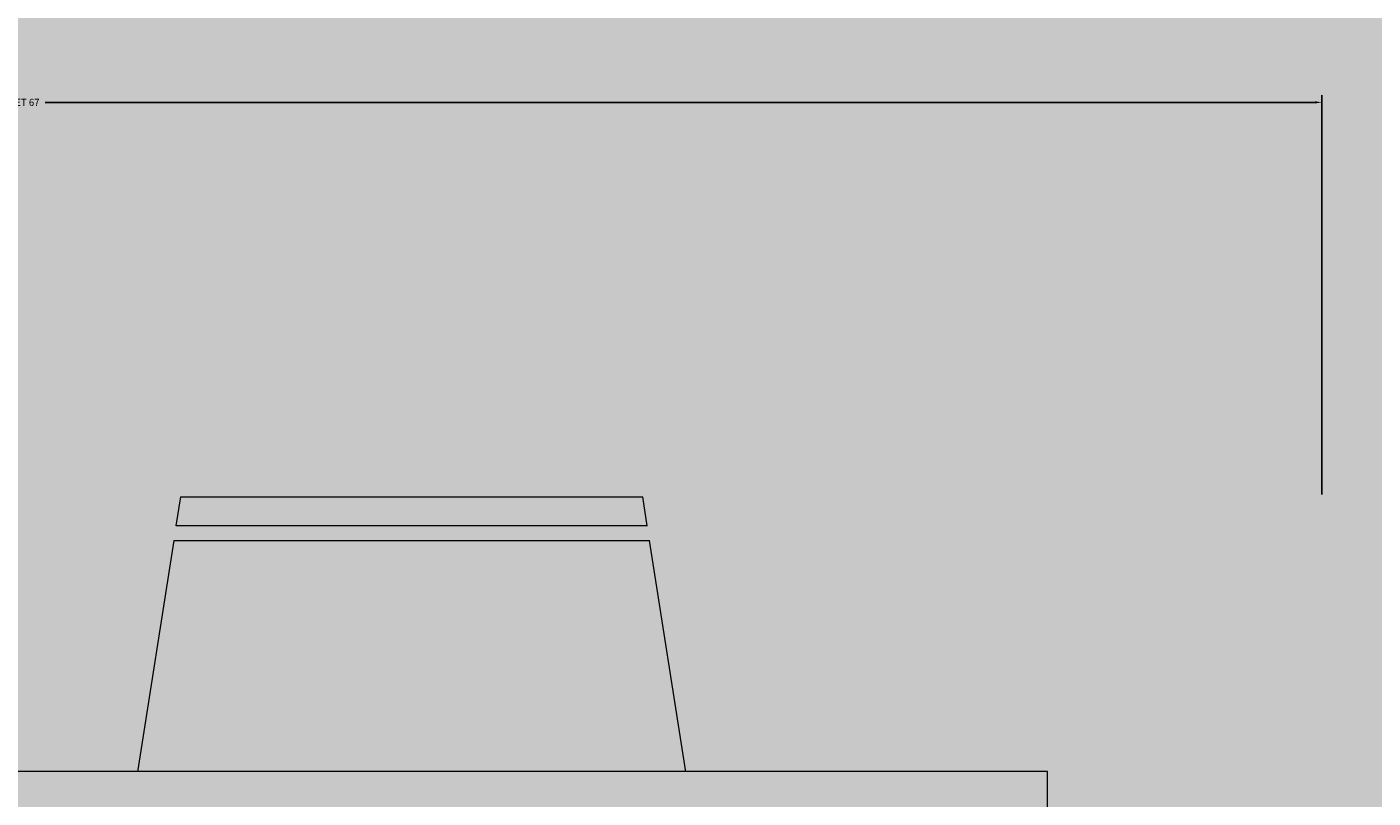
# Model space of a CAD drawing. Units: inches. Extents: x 3024 to 3952, y 1308 to 1863.
# Tile 12 of 29: x 3357 to 3392, y 1613 to 1633. Entities that reach past the tile are written whole.
import ezdxf

# ---------------------------------------------------------------- set-up
doc = ezdxf.new("R2010")
doc.units = ezdxf.units.IN
for name, color, linetype, lineweight in [('A-ANNO-DIMS', 2, 'Continuous', 18), ('A-FLOR-TILE-PATT', 7, 'Continuous', 13), ('A-FURN', 8, 'Continuous', 18), ('A-FURN-PATT', 9, 'Continuous', 13)]:
    doc.layers.add(name, color=color, linetype=linetype, lineweight=lineweight)
doc.layers.add('A-FLOR-PATT', color=254, linetype='Continuous', lineweight=13, true_color=0xfeeab9)
doc.styles.get("Standard").update_dxf_attribs({"font": 'arial.ttf'})
doc.dimstyles.get("Standard").update_dxf_attribs({"dimtxt": 0.18, "dimasz": 0.18, "dimexe": 0.18, "dimexo": 0.0625, "dimgap": 0.09, "dimtad": 0, "dimtih": 1, "dimtoh": 1, "dimdec": 4, "dimzin": 0, "dimdsep": 46, "dimtxsty": 'Standard', "dimcen": 0.09, "dimadec": 0, "dimazin": 0, "dimtfac": 1, "dimtdec": 4, "dimtofl": 0, "dimtmove": 0, "dimatfit": 3, "dimfxl": 1, "dimtolj": 1, "dimtzin": 0, "dimarcsym": 0})

# ---------------------------------------------------------------- blocks, each defined once
blk = doc.blocks.new('Dining Set - 36 x 72 in.')
for p, q in [((6, 27.5), (5.8438, 26.50042)), ((6, 27.5), (22, 27.5)), ((22.1563, 26.49966), (22, 27.5)), ((22.1584, 26.5), (5.8466, 26.5)), ((5.7657, 26.00059), (4.5153, 17.99762)), ((5.7696, 26), (22.2392, 26)), ((23.4848, 17.99762), (22.2345, 25.99926)), ((36, 18), (-36, 18)), ((36, -18), (36, 18))]:
    blk.add_line(p, q)
blk = doc.blocks.new('*D20')
at = {"layer": 'A-ANNO-DIMS', "color": 0, "lineweight": -2, "transparency": 16777216}
for p, q in [((3323.117, 1621.176), (3323.117, 1631.358)), ((3323.297, 1631.178), (3355.696, 1631.178)), ((3390.032, 1631.178), (3357.634, 1631.178)), ((3390.212, 1621.176), (3390.212, 1631.358))]:
    blk.add_line(p, q, dxfattribs=at)
at = {"layer": 'A-ANNO-DIMS', "color": 0, "transparency": 16777216}
for points in [[(3323.297, 1631.208), (3323.297, 1631.148), (3323.117, 1631.178)], [(3390.032, 1631.208), (3390.032, 1631.148), (3390.212, 1631.178)]]:
    blk.add_solid(points, dxfattribs=at)
at = {"layer": 'Defpoints', "color": 0, "transparency": 16777216}
for p in [(3390.212, 1631.178), (3323.117, 1621.114), (3390.212, 1621.114)]:
    blk.add_point(p, dxfattribs=at)
at = {"layer": 'A-ANNO-DIMS', "color": 0, "transparency": 16777216, "insert": (3356.665, 1631.178), "char_height": 0.18, "attachment_point": 5}
blk.add_mtext('\\A1;DINING SET 67', dxfattribs=at)

msp = doc.modelspace()

# ---------------------------------------------------------------- hatches: boundary and pattern name
at = {"layer": 'A-FLOR-PATT', "transparency": 33554528}
h = msp.add_hatch(color=256, dxfattribs=at)
h.dxf.hatch_style = 1
h.paths.add_polyline_path([(3460.764, 1688.6064), (3412.764, 1688.6064), (3412.764, 1694.6064), (3460.764, 1694.6064), (3460.764, 1778.6064), (3406.764, 1778.6064), (3406.764, 1759.9514), (3318.2981, 1759.9514), (3318.2981, 1658.6064), (3322.5356, 1658.6064), (3322.5356, 1652.6064), (3292.764, 1652.6064), (3292.764, 1778.6064), (3106.764, 1778.6064), (3106.764, 1628.6064), (3172.764, 1628.6064), (3172.764, 1532.6064), (3166.764, 1532.6064), (3166.764, 1628.6064), (3106.764, 1628.6064), (3106.764, 1356.8452), (3202.812, 1356.8452), (3202.812, 1354.2534), (3202.812, 1353.8388), (3202.812, 1351.1212), (3202.812, 1347.8452), (3277.764, 1347.8452), (3277.764, 1353.8452), (3277.764, 1356.8452), (3277.764, 1442.6064), (3460.764, 1442.6064)])
h.paths.add_polyline_path([(3216.238, 1527.2064), (3216.238, 1491.2064), (3214.663, 1491.2064), (3214.663, 1491.2409, -0.3966224), (3180.243, 1526.6064), (3163.0285, 1526.6064), (3163.0285, 1531.1064), (3161.716, 1531.1064), (3161.716, 1561.1064), (3163.0285, 1561.1064), (3163.0285, 1531.1064), (3163.0285, 1526.6064), (3180.243, 1526.6064, 0.3966224), (3214.663, 1491.2409), (3214.663, 1527.2064)], flags=16)
h.paths.add_polyline_path([(3227.364, 1649.8972), (3191.364, 1649.8972), (3191.364, 1651.4722), (3227.364, 1651.4722)], flags=16)
h.paths.add_polyline_path([(3323.1172, 1606.7362), (3323.8545, 1606.8514), (3323.8545, 1594.8241), (3323.1172, 1594.9393)], flags=16)
h.paths.add_polyline_path([(3324.2232, 1606.909), (3330.1216, 1607.8307), (3330.1216, 1614.1093), (3339.3495, 1614.1093), (3340.2711, 1620.0078), (3352.4136, 1620.0078), (3353.3353, 1614.1093), (3359.9941, 1614.1093), (3360.9157, 1620.0078), (3373.0582, 1620.0078), (3373.9799, 1614.1093), (3383.2077, 1614.1093), (3383.2077, 1607.8307), (3389.1062, 1606.909), (3389.1062, 1594.7665), (3383.2077, 1593.8449), (3383.2077, 1587.5663), (3373.9799, 1587.5663), (3373.0583, 1581.6678), (3360.9157, 1581.6678), (3359.9941, 1587.5663), (3353.3353, 1587.5663), (3352.4136, 1581.6678), (3340.2711, 1581.6678), (3339.3495, 1587.5663), (3330.1216, 1587.5663), (3330.1216, 1593.8449), (3324.2232, 1594.7665)], flags=16)
h.paths.add_polyline_path([(3236.1584, 1693.1064), (3236.1584, 1723.1064), (3237.4709, 1723.1064), (3237.4709, 1693.1064)], flags=16)
h.paths.add_polyline_path([(3373.2158, 1600.6847), (3373.7965, 1600.7303), (3374.3268, 1600.7874), (3374.8132, 1600.8531), (3375.2621, 1600.9247), (3375.6801, 1600.9991), (3376.0736, 1601.0735), (3376.6855, 1601.19), (3377.366, 1601.3023), (3378.0667, 1601.3814), (3378.8026, 1601.4123), (3379.5865, 1601.3839), (3380.4537, 1601.2948), (3381.301, 1601.1717), (3382.0317, 1601.0433), (3382.4398, 1600.9607), (3382.6252, 1600.9201), (3382.919, 1600.8507), (3382.9044, 1600.8531), (3382.842, 1600.8678), (3382.7541, 1600.8896), (3382.6252, 1600.9201), (3382.4398, 1600.9607), (3382.1868, 1601.0119), (3381.8738, 1601.0711), (3381.5125, 1601.1346), (3381.1149, 1601.1988), (3380.6928, 1601.2601), (3380.2581, 1601.3149), (3379.8226, 1601.3597), (3379.3984, 1601.3908), (3378.9944, 1601.4054), (3378.6092, 1601.4042), (3378.2384, 1601.3886), (3377.8777, 1601.36), (3377.5227, 1601.32), (3377.1691, 1601.2698), (3376.8127, 1601.211), (3376.4491, 1601.145), (3376.0736, 1601.0735), (3375.4177, 1600.9494), (3374.5542, 1600.8119), (3373.5044, 1600.6988)], flags=0)
h.paths.add_polyline_path([(3380.0253, 1596.7351), (3380.499, 1596.6659), (3380.9706, 1596.6119), (3381.4375, 1596.5791), (3381.8971, 1596.5736), (3382.5886, 1596.6167), (3382.7848, 1596.6692), (3382.1465, 1596.5706), (3381.236, 1596.5815), (3380.3199, 1596.6865)], flags=0)
h.paths.add_polyline_path([(3369.6414, 1603.9617), (3370.1589, 1604.0021), (3370.6218, 1604.0539), (3371.0335, 1604.1173), (3371.3978, 1604.1921), (3371.7181, 1604.2785), (3371.9984, 1604.3761), (3372.2441, 1604.483), (3372.4611, 1604.5972), (3372.655, 1604.7163), (3372.8317, 1604.8384), (3372.9968, 1604.9611), (3373.3703, 1605.2455), (3373.8426, 1605.5328), (3374.4624, 1605.7539), (3375.1058, 1605.8302), (3375.7221, 1605.8261), (3376.4109, 1605.76), (3377.1534, 1605.6376), (3377.8945, 1605.473), (3378.1382, 1605.409), (3377.7394, 1605.5074), (3377.3509, 1605.5937), (3376.9704, 1605.6677), (3376.5999, 1605.7288), (3376.2417, 1605.7762), (3375.8979, 1605.8092), (3375.5707, 1605.8271), (3375.2621, 1605.8291), (3374.9745, 1605.8146), (3374.7092, 1605.7832), (3374.4647, 1605.7359), (3374.239, 1605.6742), (3374.0298, 1605.5996), (3373.835, 1605.5134), (3373.6525, 1605.4171), (3373.4801, 1605.3123), (3373.3156, 1605.2002), (3373.1562, 1605.0825), (3372.7603, 1604.781), (3372.236, 1604.4588), (3371.5738, 1604.2283), (3370.8493, 1604.0794), (3369.9262, 1603.976)], flags=0)
h.paths.add_polyline_path([(3366.7533, 1606.5832), (3367.1713, 1606.5519), (3367.5378, 1606.5374), (3367.8568, 1606.5394), (3368.1325, 1606.5573), (3368.3694, 1606.5903), (3368.5717, 1606.6377), (3368.7438, 1606.6988), (3368.89, 1606.7728), (3369.0146, 1606.8591), (3369.121, 1606.9568), (3369.2094, 1607.0646), (3369.2792, 1607.181), (3369.3295, 1607.3046), (3369.3596, 1607.4339), (3369.3688, 1607.5676), (3369.3565, 1607.7042), (3369.3218, 1607.8422), (3369.2649, 1607.9804), (3369.1893, 1608.1187), (3369.0993, 1608.2569), (3368.9992, 1608.3952), (3368.8934, 1608.5334), (3368.7861, 1608.6717), (3368.6817, 1608.8099), (3368.4212, 1609.1804), (3368.2685, 1609.7106), (3368.4883, 1610.1814), (3369.0537, 1610.4604), (3369.6717, 1610.5097), (3370.2812, 1610.3612), (3370.4805, 1610.2968), (3370.1882, 1610.3839), (3369.9284, 1610.4472), (3369.6905, 1610.4842), (3369.4662, 1610.4933), (3369.2555, 1610.4765), (3369.0608, 1610.4367), (3368.884, 1610.3767), (3368.7274, 1610.2994), (3368.5931, 1610.2077), (3368.4833, 1610.1045), (3368.4002, 1609.9927), (3368.3451, 1609.8747), (3368.3166, 1609.7517), (3368.3127, 1609.6244), (3368.331, 1609.4935), (3368.3696, 1609.3597), (3368.4261, 1609.2237), (3368.4985, 1609.0863), (3368.5845, 1608.9482), (3368.6817, 1608.8099), (3368.7861, 1608.6717), (3368.8934, 1608.5334), (3368.9992, 1608.3952), (3369.0993, 1608.2569), (3369.3398, 1607.8876), (3369.3941, 1607.2896), (3368.9774, 1606.7817), (3368.3928, 1606.5742), (3367.7162, 1606.5303), (3367.0044, 1606.5585)], flags=0)
h.paths.add_polyline_path([(3362.1859, 1610.2589), (3362.5478, 1610.2845), (3362.8348, 1610.3275), (3363.0585, 1610.3863), (3363.2303, 1610.4595), (3363.3619, 1610.5457), (3363.463, 1610.6432), (3363.5376, 1610.7502), (3363.5876, 1610.8643), (3363.6153, 1610.9834), (3363.6229, 1611.1055), (3363.6125, 1611.2283), (3363.5861, 1611.3496), (3363.5462, 1611.4673), (3363.4949, 1611.5797), (3363.4358, 1611.6871), (3363.3723, 1611.7902), (3363.3081, 1611.8897), (3363.2468, 1611.9863), (3363.192, 1612.0808), (3363.0258, 1612.4261), (3363.3371, 1612.8672), (3363.9008, 1612.9782), (3364.4822, 1612.9641), (3365.1098, 1612.9074), (3365.328, 1612.8805), (3364.9615, 1612.9208), (3364.6426, 1612.9496), (3364.3668, 1612.9669), (3364.1299, 1612.9726), (3363.9276, 1612.9669), (3363.7555, 1612.9496), (3363.6093, 1612.9208), (3363.4848, 1612.8805), (3363.3782, 1612.8289), (3363.2889, 1612.7672), (3363.2169, 1612.6969), (3363.1622, 1612.6193), (3363.1247, 1612.5361), (3363.1046, 1612.4484), (3363.1017, 1612.358), (3363.1161, 1612.266), (3363.1472, 1612.1738), (3363.192, 1612.0808), (3363.2468, 1611.9863), (3363.3081, 1611.8897), (3363.3723, 1611.7902), (3363.4358, 1611.6871), (3363.6363, 1611.323), (3363.5979, 1610.7003), (3363.0863, 1610.3651), (3362.3983, 1610.2622)], flags=0)
h.paths.add_polyline_path([(3352.356, 1581.2991), (3352.2408, 1580.5618), (3340.4439, 1580.5618), (3340.3287, 1581.2991)], flags=16)
h.paths.add_polyline_path([(3340.4439, 1621.1137), (3352.2408, 1621.1137), (3352.356, 1620.3764), (3340.3287, 1620.3764)], flags=16)
h.paths.add_polyline_path([(3278.4282, 1504.7424), (3290.3831, 1504.7424), (3290.3831, 1502.7499), (3291.0473, 1502.7499), (3291.0473, 1494.7799), (3290.3831, 1494.7799), (3290.3831, 1494.1158), (3291.0473, 1494.1158), (3291.0473, 1486.1458), (3290.3831, 1486.1458), (3290.3831, 1484.1533), (3291.0473, 1484.1533), (3291.0473, 1483.4892, -0.0909091), (3291.0473, 1468.8776), (3291.0473, 1468.2135), (3290.3831, 1468.2135), (3290.3831, 1464.8926), (3278.4282, 1464.8926), (3278.4282, 1472.8626), (3277.764, 1473.5268), (3277.764, 1478.84), (3278.4282, 1479.5042)], flags=16)
h.paths.add_polyline_path([(3278.7603, 1504.4103), (3290.051, 1504.4103), (3290.051, 1465.2247), (3278.7603, 1465.2247)], flags=0)
h.paths.add_polyline_path([(3123.904, 1600.7821), (3117.9039, 1602.7821), (3117.9039, 1599.7821), (3119.4039, 1599.7821), (3119.4039, 1596.7821), (3118.4039, 1596.7821), (3118.4039, 1598.7821), (3117.9039, 1598.7821), (3117.9039, 1596.2821), (3109.9039, 1596.2821), (3109.9039, 1617.2821), (3117.9039, 1617.2821), (3117.9039, 1610.7821), (3123.9038, 1612.7821, -0.7025712), (3137.9039, 1606.7822, -0.7025621)], flags=16)
h.paths.add_polyline_path([(3123.9039, 1602.7822), (3123.9039, 1610.7822, -0.7345333), (3136.9039, 1606.7822, -0.7345297)], flags=0)
h.paths.add_polyline_path([(3177.972, 1689.6473), (3109.2405, 1689.6473), (3109.2405, 1741.1959), (3177.972, 1741.1959)], flags=16)
h.paths.add_polyline_path([(3373.0006, 1581.2991), (3372.8854, 1580.5618), (3361.0885, 1580.5618), (3360.9733, 1581.2991)], flags=16)
h.paths.add_polyline_path([(3361.0885, 1621.1137), (3372.8854, 1621.1137), (3373.0006, 1620.3764), (3360.9733, 1620.3764)], flags=16)
h.paths.add_polyline_path([(3116.9039, 1598.2821, -0.4142136), (3116.1539, 1597.2821), (3111.9039, 1597.2821, -0.4142136), (3110.9039, 1598.0321), (3110.9039, 1615.2821, -0.4142136), (3111.6539, 1616.2821), (3115.9039, 1616.2821, -0.4142136), (3116.9039, 1615.5321)], flags=0)
h.paths.add_polyline_path([(3121.6122, 1728.1369), (3121.6122, 1696.5205), (3110.2715, 1696.5205), (3110.2715, 1714.3906), (3121.6122, 1714.3906), (3121.6122, 1716.4526), (3110.2715, 1716.4526), (3110.2715, 1734.3228), (3123.3304, 1734.3228), (3123.3304, 1729.8552), (3134.6711, 1741.1959), (3134.6711, 1728.1369)], flags=0)
h.paths.add_polyline_path([(3389.4748, 1606.8514), (3390.2122, 1606.7362), (3390.2122, 1594.9393), (3389.4748, 1594.8241)], flags=16)
h.paths.add_polyline_path([(3257.6842, 1762.8281), (3259.6842, 1768.8281), (3256.6842, 1768.8281), (3256.6842, 1767.3281), (3253.6842, 1767.3281), (3253.6842, 1768.3281), (3255.6842, 1768.3281), (3255.6842, 1768.8281), (3253.1842, 1768.8281), (3253.1842, 1776.8281), (3274.1842, 1776.8281), (3274.1842, 1768.8281), (3267.6842, 1768.8281), (3269.6842, 1762.8282, -0.7025712), (3263.6843, 1748.8282, -0.7025621)], flags=16)
h.paths.add_polyline_path([(3259.6842, 1762.8281), (3267.6843, 1762.8281, -0.7345333), (3263.6842, 1749.8282, -0.7345297)], flags=0)
h.paths.add_polyline_path([(3411.264, 1715.6064), (3411.264, 1716.9189), (3441.264, 1716.9189), (3441.264, 1715.6064)], flags=16)
h.paths.add_polyline_path([(3178.3806, 1449.1876), (3178.3806, 1397.639), (3109.6491, 1397.639), (3109.6491, 1449.1876)], flags=16)
h.paths.add_polyline_path([(3397.1501, 1541.7146), (3419.6183, 1541.7146), (3419.6183, 1496.7783), (3397.1501, 1496.7783)], flags=16)
h.paths.add_polyline_path([(3254.1842, 1770.5781), (3254.1842, 1774.8281, -0.4142136), (3254.9342, 1775.8281), (3272.1842, 1775.8281, -0.4142136), (3273.1842, 1775.0781), (3273.1842, 1770.8281, -0.4142136), (3272.4342, 1769.8281), (3255.1842, 1769.8281, -0.4142136)], flags=0)
h.paths.add_polyline_path([(3403.672, 1500.7601), (3403.6016, 1500.3997), (3403.5328, 1500.0441), (3403.4662, 1499.6867), (3403.4027, 1499.3226), (3403.3464, 1498.9532), (3403.3025, 1498.5811), (3403.2759, 1498.2091), (3403.2714, 1497.8401), (3403.3064, 1497.2813), (3403.3491, 1497.1219), (3403.2689, 1497.6395), (3403.2778, 1498.3719), (3403.3635, 1499.0984), (3403.4889, 1499.8168), (3403.6016, 1500.3997), (3403.672, 1500.7601), (3403.744, 1501.1315), (3403.817, 1501.5205), (3403.891, 1501.9336), (3403.9656, 1502.3769), (3404.0404, 1502.8572), (3404.115, 1503.3786), (3404.2264, 1504.2311), (3404.2571, 1504.5223), (3404.1552, 1503.6598), (3404.0063, 1502.6193), (3403.8604, 1501.7518), (3403.744, 1501.1315)], flags=0)
h.paths.add_polyline_path([(3406.5868, 1505.0416), (3406.6121, 1504.5236), (3406.6492, 1504.0526), (3406.6956, 1503.624), (3406.7491, 1503.2333), (3406.8072, 1502.8759), (3406.8676, 1502.5473), (3406.9281, 1502.243), (3407.0268, 1501.7597), (3407.1416, 1501.1368), (3407.2087, 1500.3904), (3407.1804, 1499.6703), (3407.1078, 1498.9956), (3407.0074, 1498.3199), (3406.8809, 1497.6059), (3406.7403, 1496.9627), (3406.7418, 1496.9824), (3406.7491, 1497.0249), (3406.8229, 1497.3409), (3406.8364, 1497.4025), (3406.878, 1497.6078), (3406.9261, 1497.8614), (3406.9777, 1498.1526), (3407.0298, 1498.4712), (3407.0797, 1498.8068), (3407.1243, 1499.149), (3407.1607, 1499.4874), (3407.1859, 1499.8115), (3407.1978, 1500.1137), (3407.1969, 1500.3962), (3407.1841, 1500.6642), (3407.1609, 1500.9225), (3407.1284, 1501.1761), (3407.0876, 1501.43), (3407.0398, 1501.6891), (3406.9862, 1501.9585), (3406.8832, 1502.4628), (3406.7712, 1503.0713), (3406.6657, 1503.8424), (3406.5924, 1504.7735)], flags=0)
h.paths.add_polyline_path([(3409.2517, 1507.8962), (3409.2752, 1507.4282), (3409.3079, 1507.0076), (3409.3501, 1506.6314), (3409.4015, 1506.2969), (3409.4624, 1506.0009), (3409.5326, 1505.7406), (3409.6119, 1505.5128), (3409.6988, 1505.3131), (3409.7915, 1505.1368), (3409.8883, 1504.9792), (3409.9875, 1504.8356), (3410.0872, 1504.7015), (3410.1859, 1504.572), (3410.4508, 1504.2132), (3410.7205, 1503.6035), (3410.8059, 1502.8824), (3410.7619, 1502.0875), (3410.6122, 1501.2299), (3410.4402, 1500.6169), (3410.2538, 1500.0031), (3410.0536, 1499.3219), (3409.9909, 1499.0812), (3410.1761, 1499.7472), (3410.3596, 1500.3513), (3410.4512, 1500.6561), (3410.5312, 1500.9412), (3410.6013, 1501.226), (3410.6614, 1501.512), (3410.7111, 1501.7964), (3410.7496, 1502.0763), (3410.7764, 1502.3489), (3410.7909, 1502.6114), (3410.7926, 1502.8608), (3410.7808, 1503.0944), (3410.7553, 1503.31), (3410.7169, 1503.5087), (3410.6667, 1503.6921), (3410.6061, 1503.8621), (3410.5361, 1504.0203), (3410.4578, 1504.1686), (3410.3726, 1504.3088), (3410.2815, 1504.4424), (3410.1859, 1504.572), (3410.0872, 1504.7015), (3409.859, 1505.0083), (3409.5943, 1505.5117), (3409.4266, 1506.1336), (3409.324, 1506.8011), (3409.2586, 1507.6407)], flags=0)
h.paths.add_polyline_path([(3411.4914, 1510.5878), (3411.4432, 1510.1586), (3411.4054, 1509.775), (3411.38, 1509.4354), (3411.3681, 1509.1376), (3411.3698, 1508.8784), (3411.3843, 1508.6542), (3411.4112, 1508.4618), (3411.4497, 1508.2974), (3411.4994, 1508.1575), (3411.5595, 1508.0388), (3411.6296, 1507.9375), (3411.7097, 1507.851), (3411.802, 1507.7792), (3411.9096, 1507.7225), (3412.0353, 1507.6817), (3412.1821, 1507.6572), (3412.3528, 1507.6496), (3412.5505, 1507.6597), (3412.778, 1507.6879), (3413.0364, 1507.7341), (3413.3194, 1507.7955), (3413.6188, 1507.8687), (3413.9264, 1507.95), (3414.234, 1508.036), (3414.5333, 1508.1232), (3414.8163, 1508.208), (3415.0747, 1508.287), (3415.3023, 1508.3569), (3415.5007, 1508.4158), (3415.6733, 1508.4617), (3416.1158, 1508.5538), (3416.512, 1508.2591), (3416.716, 1507.6581), (3416.61, 1507.0003), (3416.3052, 1506.3411), (3415.8928, 1505.618), (3415.7339, 1505.3633), (3415.9914, 1505.791), (3416.201, 1506.1583), (3416.3666, 1506.4739), (3416.4925, 1506.7462), (3416.5828, 1506.9838), (3416.6413, 1507.1949), (3416.6725, 1507.3883), (3416.6799, 1507.5705), (3416.6662, 1507.7417), (3416.6339, 1507.9), (3416.5851, 1508.0436), (3416.5223, 1508.1709), (3416.4478, 1508.28), (3416.3639, 1508.3692), (3416.273, 1508.4368), (3416.1765, 1508.4815), (3416.0718, 1508.5047), (3415.9553, 1508.5079), (3415.8237, 1508.493), (3415.6733, 1508.4617), (3415.5007, 1508.4158), (3415.3327, 1508.3659), (3414.6495, 1508.157), (3414.0606, 1507.9855), (3413.4456, 1507.8229), (3412.8838, 1507.701), (3412.5505, 1507.6597), (3412.0748, 1507.6354), (3411.595, 1507.8883), (3411.398, 1508.4429), (3411.3624, 1508.9927), (3411.3854, 1509.5711), (3411.4578, 1510.3071)], flags=0)
h.paths.add_polyline_path([(3135.0797, 1449.1876), (3135.0797, 1436.1286), (3122.0208, 1436.1286), (3122.0208, 1404.5122), (3110.6801, 1404.5122), (3110.6801, 1422.3823), (3122.0208, 1422.3823), (3122.0208, 1424.4443), (3110.6801, 1424.4443), (3110.6801, 1442.3145), (3123.739, 1442.3145), (3123.739, 1437.8469)], flags=0)
h.paths.add_polyline_path([(3416.4944, 1514.2949), (3416.4837, 1513.8511), (3416.4893, 1513.4867), (3416.5102, 1513.1926), (3416.5451, 1512.9593), (3416.5929, 1512.7775), (3416.6524, 1512.6379), (3416.7224, 1512.531), (3416.8017, 1512.4488), (3416.8886, 1512.3882), (3416.9813, 1512.3476), (3417.0781, 1512.3251), (3417.1773, 1512.3189), (3417.277, 1512.3274), (3417.3757, 1512.3488), (3417.4713, 1512.3813), (3417.5627, 1512.4229), (3417.65, 1512.471), (3417.7338, 1512.5225), (3417.8146, 1512.5747), (3417.8931, 1512.6245), (3417.9699, 1512.6691), (3418.2968, 1512.8265), (3418.6505, 1512.4645), (3418.7037, 1511.9342), (3418.6693, 1511.3839), (3418.6076, 1510.8228), (3418.5777, 1510.5927), (3418.6197, 1510.9333), (3418.6525, 1511.2311), (3418.6759, 1511.4903), (3418.6899, 1511.7144), (3418.6946, 1511.9069), (3418.6899, 1512.0713), (3418.6759, 1512.2112), (3418.6525, 1512.33), (3418.6197, 1512.4311), (3418.5778, 1512.5177), (3418.5276, 1512.5903), (3418.4705, 1512.6488), (3418.4075, 1512.6933), (3418.3399, 1512.7237), (3418.2686, 1512.7401), (3418.1951, 1512.7424), (3418.1204, 1512.7307), (3418.0455, 1512.7055), (3417.9792, 1512.6736), (3417.65, 1512.471), (3417.5627, 1512.4229), (3417.4713, 1512.3813), (3417.3757, 1512.3488), (3417.277, 1512.3274), (3416.878, 1512.2936), (3416.5757, 1512.7549), (3416.492, 1513.3145), (3416.4808, 1514.0384)], flags=0)
h.paths.add_polyline_path([(3392.8223, 1481.9454), (3396.7707, 1481.9454), (3396.7707, 1480.9201), (3428.3585, 1480.9201), (3428.3585, 1481.9454), (3432.3069, 1481.9454), (3432.3069, 1464.8354, -0.266667), (3392.8223, 1464.8354)], flags=16)
h.paths.add_polyline_path([(3431.203, 1547.5428), (3450.8613, 1547.5428, -0.1904762), (3450.8614, 1484.031), (3431.203, 1484.031), (3431.203, 1488.5675), (3432.3809, 1488.5675), (3432.3809, 1543.0062), (3431.203, 1543.0062)], flags=16)
h.paths.add_polyline_path([(3451.9233, 1524.86, -0.0496282), (3451.9233, 1506.7138), (3446.7921, 1506.7138), (3446.7921, 1524.86)], flags=0)
h.paths.add_polyline_path([(3460.764, 1436.6064), (3277.764, 1436.6064), (3277.764, 1356.8452), (3277.764, 1353.8452), (3460.764, 1353.8452)], flags=17)
h.paths.add_polyline_path([(3121.3033, 1577.378), (3153.693, 1577.378), (3153.693, 1586.6752), (3121.3033, 1586.6752)], flags=24)
h.paths.add_polyline_path([(3164.1457, 1464.1276), (3210.4801, 1464.1276), (3210.4801, 1473.4247), (3164.1457, 1473.4247)], flags=24)
h.paths.add_polyline_path([(3343.1909, 1505.8863), (3373.7236, 1505.8863), (3373.7236, 1515.1773), (3343.1909, 1515.1773)], flags=24)
h.paths.add_polyline_path([(3337.6353, 1564.2926), (3370.0189, 1564.2926), (3370.0189, 1573.5836), (3337.6353, 1573.5836)], flags=24)
h.paths.add_polyline_path([(3419.204, 1753.8578), (3453.3997, 1753.8578), (3453.3997, 1762.9956), (3419.204, 1762.9956)], flags=24)
h.paths.add_polyline_path([(3341.2523, 1701.0246), (3381.0761, 1701.0246), (3381.0761, 1710.3156), (3341.2523, 1710.3156)], flags=24)
h.paths.add_polyline_path([(3245.8895, 1726.2997), (3278.2793, 1726.2997), (3278.2793, 1735.5968), (3245.8895, 1735.5968)], flags=24)
h.paths.add_polyline_path([(3128.8045, 1668.6736), (3175.1389, 1668.6736), (3175.1389, 1677.9707), (3128.8045, 1677.9707)], flags=24)
h.paths.add_polyline_path([(3345.9997, 1396.0062), (3389.09, 1396.0062), (3389.09, 1405.3033), (3345.9997, 1405.3033)], flags=24)
at = {"layer": 'A-FLOR-TILE-PATT', "transparency": 33554569}
h = msp.add_hatch(dxfattribs=at)
h.set_pattern_fill('ANGLE', color=256, scale=2)
h.set_pattern_definition([(0, (0, 0), (0, 13.97), [10.16, -3.81]), (90, (0, 0), (-13.97, 9e-16), [10.16, -3.81])])
h.paths.add_polyline_path([(3292.764, 1778.6064), (3232.764, 1778.6064), (3232.764, 1694.6064), (3236.1584, 1694.6064), (3236.1584, 1723.1064), (3237.4709, 1723.1064), (3237.4709, 1723.0777, -0.3870039), (3266.1209, 1694.6064), (3292.764, 1694.6064)])
h.paths.add_polyline_path([(3263.6843, 1748.8282, -0.7025621), (3257.6842, 1762.8281), (3259.6842, 1768.8281), (3256.6842, 1768.8281), (3256.6842, 1767.3281), (3253.6842, 1767.3281), (3253.6842, 1768.3281), (3255.6842, 1768.3281), (3255.6842, 1768.8281), (3253.1842, 1768.8281), (3253.1842, 1776.8281), (3274.1842, 1776.8281), (3274.1842, 1768.8281), (3267.6842, 1768.8281), (3269.6842, 1762.8282, -0.7025712)], flags=16)
h.paths.add_polyline_path([(3263.6842, 1749.8282, -0.7345297), (3259.6842, 1762.8281), (3267.6843, 1762.8281, -0.7345333)], flags=0)
h.paths.add_polyline_path([(3255.1842, 1769.8281, -0.4142136), (3254.1842, 1770.5781), (3254.1842, 1774.8281, -0.4142136), (3254.9342, 1775.8281), (3272.1842, 1775.8281, -0.4142136), (3273.1842, 1775.0781), (3273.1842, 1770.8281, -0.4142136), (3272.4342, 1769.8281)], flags=0)
h.paths.add_polyline_path([(3460.764, 1436.6064), (3277.764, 1436.6064), (3277.764, 1356.8452), (3277.764, 1353.8452), (3460.764, 1353.8452)])
h.paths.add_polyline_path([(3166.764, 1628.6064), (3106.764, 1628.6064), (3106.764, 1532.6064), (3133.066, 1532.6064, -0.3870039), (3161.716, 1561.0777), (3161.716, 1561.1064), (3163.0285, 1561.1064), (3163.0285, 1532.6064), (3166.764, 1532.6064)])
h.paths.add_polyline_path([(3123.904, 1600.7821), (3117.9039, 1602.7821), (3117.9039, 1599.7821), (3119.4039, 1599.7821), (3119.4039, 1596.7821), (3118.4039, 1596.7821), (3118.4039, 1598.7821), (3117.9039, 1598.7821), (3117.9039, 1596.2821), (3109.9039, 1596.2821), (3109.9039, 1617.2821), (3117.9039, 1617.2821), (3117.9039, 1610.7821), (3123.9038, 1612.7821, -0.7025712), (3137.9039, 1606.7822, -0.7025621)], flags=16)
h.paths.add_polyline_path([(3123.9039, 1602.7822), (3123.9039, 1610.7822, -0.7345333), (3136.9039, 1606.7822, -0.7345297)], flags=0)
h.paths.add_polyline_path([(3116.1539, 1597.2821), (3111.9039, 1597.2821, -0.4142136), (3110.9039, 1598.0321), (3110.9039, 1615.2821, -0.4142136), (3111.6539, 1616.2821), (3115.9039, 1616.2821, -0.4142136), (3116.9039, 1615.5321), (3116.9039, 1598.2821, -0.4142136)], flags=0)
h.paths.add_polyline_path([(3245.8895, 1726.2997), (3278.2793, 1726.2997), (3278.2793, 1735.5968), (3245.8895, 1735.5968)], flags=24)
h.paths.add_polyline_path([(3345.9997, 1396.0062), (3389.09, 1396.0062), (3389.09, 1405.3033), (3345.9997, 1405.3033)], flags=24)
h.paths.add_polyline_path([(3121.3033, 1577.378), (3153.693, 1577.378), (3153.693, 1586.6752), (3121.3033, 1586.6752)], flags=24)
at = {"layer": 'A-FURN-PATT', "transparency": 33554511}
h = msp.add_hatch(color=256, dxfattribs=at)
h.dxf.hatch_style = 1
h.paths.add_polyline_path([(3373.0582, 1620.0078), (3360.9157, 1620.0078), (3359.9941, 1614.1093), (3373.9799, 1614.1093)])
h.paths.add_polyline_path([(3372.8854, 1621.1137), (3361.0885, 1621.1137), (3360.9733, 1620.3764), (3373.0006, 1620.3764)])
h.paths.add_polyline_path([(3389.1062, 1606.909), (3383.2077, 1607.8307), (3383.2077, 1593.8449), (3389.1062, 1594.7665)])
h.paths.add_polyline_path([(3390.2122, 1606.7362), (3389.4748, 1606.8514), (3389.4748, 1594.8241), (3390.2122, 1594.9393)])
h.paths.add_polyline_path([(3373.9799, 1587.5663), (3359.9941, 1587.5663), (3360.9157, 1581.6678), (3373.0583, 1581.6678)])
h.paths.add_polyline_path([(3373.0006, 1581.2991), (3360.9733, 1581.2991), (3361.0885, 1580.5618), (3372.8854, 1580.5618)])
h.paths.add_polyline_path([(3353.3353, 1587.5663), (3339.3495, 1587.5663), (3340.2711, 1581.6678), (3352.4136, 1581.6678)])
h.paths.add_polyline_path([(3352.356, 1581.2991), (3340.3287, 1581.2991), (3340.4439, 1580.5618), (3352.2408, 1580.5618)])
h.paths.add_polyline_path([(3330.1216, 1607.8307), (3324.2232, 1606.909), (3324.2232, 1594.7665), (3330.1216, 1593.8449)])
h.paths.add_polyline_path([(3323.8545, 1606.8514), (3323.1172, 1606.7362), (3323.1172, 1594.9393), (3323.8545, 1594.8241)])
h.paths.add_polyline_path([(3352.4136, 1620.0078), (3340.2711, 1620.0078), (3339.3495, 1614.1093), (3353.3353, 1614.1093)])
h.paths.add_polyline_path([(3352.2408, 1621.1137), (3340.4439, 1621.1137), (3340.3287, 1620.3764), (3352.356, 1620.3764)])
at = {"layer": 'A-FURN-PATT', "transparency": 33554600}
h = msp.add_hatch(color=256, dxfattribs=at)
h.dxf.hatch_style = 1
h.paths.add_polyline_path([(3363.5462, 1611.4673), (3363.4949, 1611.5797), (3363.4358, 1611.6871), (3363.3723, 1611.7902), (3363.2557, 1611.9708), (3363.16, 1612.1359), (3363.1003, 1612.3129), (3363.1061, 1612.4946), (3363.1815, 1612.6623), (3363.3264, 1612.8038), (3363.5397, 1612.9071), (3363.7555, 1612.9496), (3363.9276, 1612.9669), (3364.1299, 1612.9726), (3364.3668, 1612.9669), (3364.6426, 1612.9496), (3364.9615, 1612.9208), (3365.328, 1612.8805), (3365.7471, 1612.8287), (3366.2271, 1612.7662), (3366.7769, 1612.6936), (3367.4055, 1612.6117), (3368.1221, 1612.5211), (3368.9354, 1612.4225), (3369.8546, 1612.3168), (3370.8886, 1612.2046), (3372.0442, 1612.0866), (3373.3189, 1611.9636), (3374.7081, 1611.8363), (3376.2072, 1611.7054), (3377.8113, 1611.5716), (3379.516, 1611.4356), (3381.3163, 1611.2982), (3383.2077, 1611.1601), (3383.2077, 1614.1093), (3330.1216, 1614.1093), (3330.1216, 1611.8974), (3333.6775, 1611.8808), (3336.899, 1611.834), (3339.8144, 1611.7613), (3342.4523, 1611.667), (3344.8411, 1611.5554), (3347.0091, 1611.4308), (3348.985, 1611.2976), (3350.797, 1611.1601), (3352.4691, 1611.0223), (3354.0078, 1610.8874), (3355.4146, 1610.7583), (3356.6916, 1610.6378), (3357.8403, 1610.5289), (3358.8627, 1610.4343), (3359.7605, 1610.357), (3360.5355, 1610.2999), (3361.1912, 1610.2651), (3361.7375, 1610.2519), (3362.1859, 1610.2589), (3362.5478, 1610.2845), (3362.8348, 1610.3275), (3363.0585, 1610.3863), (3363.2303, 1610.4595), (3363.3619, 1610.5457), (3363.463, 1610.6432), (3363.5376, 1610.7502), (3363.5876, 1610.8643), (3363.6153, 1610.9834), (3363.6229, 1611.1055), (3363.6125, 1611.2283), (3363.5861, 1611.3496)])
h.paths.add_polyline_path([(3368.8934, 1608.5334), (3368.7093, 1608.7706), (3368.5315, 1609.0235), (3368.3879, 1609.2961), (3368.3108, 1609.5637), (3368.3187, 1609.8182), (3368.4002, 1609.9927), (3368.4833, 1610.1045), (3368.5931, 1610.2077), (3368.7274, 1610.2994), (3368.884, 1610.3767), (3369.0608, 1610.4367), (3369.2555, 1610.4765), (3369.4662, 1610.4933), (3369.6905, 1610.4842), (3369.9284, 1610.4472), (3370.1882, 1610.3839), (3370.4805, 1610.2968), (3370.8156, 1610.1885), (3371.204, 1610.0615), (3371.6561, 1609.9183), (3372.1824, 1609.7614), (3372.7933, 1609.5933), (3373.5016, 1609.4153), (3374.3298, 1609.2232), (3375.3028, 1609.0117), (3376.4453, 1608.7754), (3377.7822, 1608.5088), (3379.3383, 1608.2065), (3381.1386, 1607.8633), (3383.2077, 1607.4735), (3383.2077, 1611.1601), (3381.3163, 1611.2982), (3379.516, 1611.4356), (3377.8113, 1611.5716), (3376.2072, 1611.7054), (3374.7081, 1611.8363), (3373.3189, 1611.9636), (3372.0442, 1612.0866), (3370.8886, 1612.2046), (3369.8546, 1612.3168), (3368.9354, 1612.4225), (3368.1221, 1612.5211), (3367.4055, 1612.6117), (3366.7769, 1612.6936), (3366.2271, 1612.7662), (3365.7471, 1612.8287), (3365.328, 1612.8805), (3364.9615, 1612.9208), (3364.6426, 1612.9496), (3364.3668, 1612.9669), (3364.1299, 1612.9726), (3363.9276, 1612.9669), (3363.7555, 1612.9496), (3363.6093, 1612.9208), (3363.4848, 1612.8805), (3363.3782, 1612.8289), (3363.2889, 1612.7672), (3363.2169, 1612.6969), (3363.1622, 1612.6193), (3363.1247, 1612.5361), (3363.1046, 1612.4484), (3363.1017, 1612.358), (3363.1161, 1612.266), (3363.1472, 1612.1738), (3363.192, 1612.0808), (3363.2468, 1611.9863), (3363.3081, 1611.8897), (3363.4181, 1611.7194), (3363.529, 1611.5178), (3363.6075, 1611.2866), (3363.6284, 1611.0397), (3363.5728, 1610.8008), (3363.4229, 1610.5856), (3363.2303, 1610.4595), (3363.0585, 1610.3863), (3362.8348, 1610.3275), (3362.5478, 1610.2845), (3362.1859, 1610.2589), (3361.7375, 1610.2519), (3361.1912, 1610.2651), (3360.5355, 1610.2999), (3359.7605, 1610.357), (3358.8627, 1610.4343), (3357.8403, 1610.5289), (3356.6916, 1610.6378), (3355.4146, 1610.7583), (3354.0078, 1610.8874), (3352.4691, 1611.0223), (3350.797, 1611.1601), (3348.985, 1611.2976), (3347.0091, 1611.4308), (3344.8411, 1611.5554), (3342.4523, 1611.667), (3339.8144, 1611.7613), (3336.899, 1611.834), (3333.6775, 1611.8808), (3330.1216, 1611.8974), (3330.1216, 1608.2109), (3335.3, 1608.3161), (3339.5794, 1608.3616), (3343.0805, 1608.3567), (3345.9238, 1608.3107), (3348.23, 1608.2331), (3350.1196, 1608.1331), (3351.7134, 1608.0202), (3353.1317, 1607.9036), (3354.475, 1607.7912), (3355.7618, 1607.6838), (3356.9902, 1607.5807), (3358.1585, 1607.4812), (3359.2649, 1607.3846), (3360.3076, 1607.2902), (3361.2846, 1607.1972), (3362.1945, 1607.1049), (3363.0358, 1607.0131), (3363.8102, 1606.9234), (3364.5198, 1606.8381), (3365.1667, 1606.7593), (3365.7532, 1606.6891), (3366.2814, 1606.6297), (3366.7533, 1606.5832), (3367.1713, 1606.5519), (3367.5378, 1606.5374), (3367.8568, 1606.5394), (3368.1325, 1606.5573), (3368.3694, 1606.5903), (3368.5717, 1606.6377), (3368.7438, 1606.6988), (3368.89, 1606.7728), (3369.0146, 1606.8591), (3369.121, 1606.9568), (3369.2094, 1607.0646), (3369.2792, 1607.181), (3369.3295, 1607.3046), (3369.3596, 1607.4339), (3369.3688, 1607.5676), (3369.3565, 1607.7042), (3369.3218, 1607.8422), (3369.2649, 1607.9804), (3369.1893, 1608.1187), (3369.0993, 1608.2569), (3368.9992, 1608.3952)])
h.paths.add_polyline_path([(3374.239, 1605.6742), (3374.4647, 1605.7359), (3374.7092, 1605.7832), (3374.9745, 1605.8146), (3375.2621, 1605.8291), (3375.5707, 1605.8271), (3375.8979, 1605.8092), (3376.2417, 1605.7762), (3376.5999, 1605.7288), (3376.9704, 1605.6677), (3377.3509, 1605.5937), (3377.7394, 1605.5074), (3378.1382, 1605.409), (3378.5679, 1605.2962), (3379.0538, 1605.1661), (3379.621, 1605.0159), (3380.2949, 1604.8426), (3381.1005, 1604.6434), (3382.0631, 1604.4154), (3383.2077, 1604.1557), (3383.2077, 1607.4735), (3381.1386, 1607.8633), (3379.3383, 1608.2065), (3377.7822, 1608.5088), (3376.4453, 1608.7754), (3375.3028, 1609.0117), (3374.3298, 1609.2232), (3373.5016, 1609.4153), (3372.7933, 1609.5933), (3372.1824, 1609.7614), (3371.6561, 1609.9183), (3371.204, 1610.0615), (3370.8156, 1610.1885), (3370.4805, 1610.2968), (3370.1882, 1610.3839), (3369.9284, 1610.4472), (3369.6905, 1610.4842), (3369.4662, 1610.4933), (3369.2555, 1610.4765), (3369.0608, 1610.4367), (3368.884, 1610.3767), (3368.7274, 1610.2994), (3368.5931, 1610.2077), (3368.4833, 1610.1045), (3368.4002, 1609.9927), (3368.3451, 1609.8747), (3368.3166, 1609.7517), (3368.3127, 1609.6244), (3368.331, 1609.4935), (3368.3696, 1609.3597), (3368.4261, 1609.2237), (3368.4985, 1609.0863), (3368.5845, 1608.9482), (3368.6817, 1608.8099), (3368.7861, 1608.6717), (3368.9798, 1608.422), (3369.1584, 1608.1753), (3369.306, 1607.9053), (3369.3736, 1607.6361), (3369.355, 1607.3674), (3369.2539, 1607.1187), (3369.121, 1606.9568), (3369.0146, 1606.8591), (3368.89, 1606.7728), (3368.7438, 1606.6988), (3368.5717, 1606.6377), (3368.3694, 1606.5903), (3368.1325, 1606.5573), (3367.8568, 1606.5394), (3367.5378, 1606.5374), (3367.1713, 1606.5519), (3366.7533, 1606.5832), (3366.2814, 1606.6297), (3365.7532, 1606.6891), (3365.1667, 1606.7593), (3364.5198, 1606.8381), (3363.8102, 1606.9234), (3363.0358, 1607.0131), (3362.1945, 1607.1049), (3361.2846, 1607.1972), (3360.3076, 1607.2902), (3359.2649, 1607.3846), (3358.1585, 1607.4812), (3356.9902, 1607.5807), (3355.7618, 1607.6838), (3354.475, 1607.7912), (3353.1317, 1607.9036), (3351.7134, 1608.0202), (3350.1196, 1608.1331), (3348.23, 1608.2331), (3345.9238, 1608.3107), (3343.0805, 1608.3567), (3339.5794, 1608.3616), (3335.3, 1608.3161), (3330.1216, 1608.2109), (3330.1216, 1604.893), (3334.0178, 1604.7712), (3337.4438, 1604.6789), (3340.4479, 1604.6111), (3343.0782, 1604.5627), (3345.3832, 1604.5288), (3347.4109, 1604.5042), (3349.2096, 1604.4839), (3350.8276, 1604.4629), (3352.3079, 1604.4371), (3353.6722, 1604.4062), (3354.9372, 1604.3711), (3356.1194, 1604.3323), (3357.2353, 1604.2907), (3358.3015, 1604.2469), (3359.3347, 1604.2016), (3360.3512, 1604.1557), (3361.3635, 1604.1098), (3362.3673, 1604.0654), (3363.3537, 1604.0239), (3364.3142, 1603.9867), (3365.2402, 1603.9553), (3366.1229, 1603.931), (3366.9539, 1603.9154), (3367.7243, 1603.9099), (3368.4277, 1603.9157), (3369.0654, 1603.9329), (3369.6414, 1603.9617), (3370.1589, 1604.0021), (3370.6218, 1604.0539), (3371.0335, 1604.1173), (3371.3978, 1604.1921), (3371.7181, 1604.2785), (3371.9984, 1604.3761), (3372.2441, 1604.483), (3372.4611, 1604.5972), (3372.655, 1604.7163), (3372.8317, 1604.8384), (3372.9968, 1604.9611), (3373.2698, 1605.169), (3373.4801, 1605.3123), (3373.6525, 1605.4171), (3373.835, 1605.5134), (3374.0298, 1605.5996)])
h.paths.add_polyline_path([(3383.2077, 1604.1557), (3382.0631, 1604.4154), (3381.1005, 1604.6434), (3380.2949, 1604.8426), (3379.621, 1605.0159), (3379.0538, 1605.1661), (3378.5679, 1605.2962), (3378.1382, 1605.409), (3377.7394, 1605.5074), (3377.3509, 1605.5937), (3376.9704, 1605.6677), (3376.5999, 1605.7288), (3376.2417, 1605.7762), (3375.8979, 1605.8092), (3375.5707, 1605.8271), (3375.2621, 1605.8291), (3374.9745, 1605.8146), (3374.7092, 1605.7832), (3374.4647, 1605.7359), (3374.239, 1605.6742), (3374.0298, 1605.5996), (3373.835, 1605.5134), (3373.6525, 1605.4171), (3373.4801, 1605.3123), (3373.3156, 1605.2002), (3373.1562, 1605.0825), (3372.9968, 1604.9611), (3372.8317, 1604.8384), (3372.655, 1604.7163), (3372.4611, 1604.5972), (3372.2441, 1604.483), (3371.9984, 1604.3761), (3371.7181, 1604.2785), (3371.3978, 1604.1921), (3371.0335, 1604.1173), (3370.6218, 1604.0539), (3370.1589, 1604.0021), (3369.6414, 1603.9617), (3369.0654, 1603.9329), (3368.4277, 1603.9157), (3367.7243, 1603.9099), (3366.9539, 1603.9154), (3366.1229, 1603.931), (3365.2402, 1603.9553), (3364.3142, 1603.9867), (3363.3537, 1604.0239), (3362.3673, 1604.0654), (3361.3635, 1604.1098), (3360.3512, 1604.1557), (3359.3347, 1604.2016), (3358.3015, 1604.2469), (3357.2353, 1604.2907), (3356.1194, 1604.3323), (3354.9372, 1604.3711), (3353.6722, 1604.4062), (3352.3079, 1604.4371), (3350.8276, 1604.4629), (3349.2096, 1604.4839), (3347.4109, 1604.5042), (3345.3832, 1604.5288), (3343.0782, 1604.5627), (3340.4479, 1604.6111), (3337.4438, 1604.6789), (3334.0178, 1604.7712), (3330.1216, 1604.893), (3330.1216, 1600.1005), (3333.9619, 1600.3518), (3337.4803, 1600.556), (3340.7006, 1600.7177), (3343.6466, 1600.8416), (3346.342, 1600.9324), (3348.8107, 1600.9947), (3351.0762, 1601.0333), (3353.1625, 1601.0528), (3355.0913, 1601.0575), (3356.8769, 1601.0495), (3358.5313, 1601.0307), (3360.0671, 1601.0029), (3361.4962, 1600.9679), (3362.831, 1600.9275), (3364.0837, 1600.8836), (3365.2666, 1600.8378), (3366.3897, 1600.7921), (3367.4545, 1600.7485), (3368.4603, 1600.7093), (3369.4063, 1600.6765), (3370.2918, 1600.6524), (3371.1161, 1600.6391), (3371.8785, 1600.6387), (3372.5783, 1600.6535), (3373.2158, 1600.6847), (3373.7965, 1600.7303), (3374.3268, 1600.7874), (3374.8132, 1600.8531), (3375.2621, 1600.9247), (3375.6801, 1600.9991), (3376.0736, 1601.0735), (3376.4491, 1601.145), (3376.8127, 1601.211), (3377.1691, 1601.2698), (3377.5227, 1601.32), (3377.8777, 1601.36), (3378.2384, 1601.3886), (3378.6092, 1601.4042), (3378.9944, 1601.4054), (3379.3984, 1601.3908), (3379.8226, 1601.3597), (3380.2581, 1601.3149), (3380.6928, 1601.2601), (3381.1149, 1601.1988), (3381.5125, 1601.1346), (3381.8738, 1601.0711), (3382.1868, 1601.0119), (3382.4398, 1600.9607), (3382.6252, 1600.9201), (3382.7541, 1600.8896), (3382.842, 1600.8678), (3382.9044, 1600.8531), (3382.9566, 1600.8443), (3383.0143, 1600.8397), (3383.0929, 1600.838), (3383.2077, 1600.8378)])
h.paths.add_polyline_path([(3383.2077, 1600.8378), (3382.9677, 1600.8383), (3382.842, 1600.8678), (3382.7541, 1600.8896), (3382.6252, 1600.9201), (3382.4398, 1600.9607), (3382.1868, 1601.0119), (3381.8738, 1601.0711), (3381.5125, 1601.1346), (3381.1149, 1601.1988), (3380.6928, 1601.2601), (3380.2581, 1601.3149), (3379.8226, 1601.3597), (3379.3984, 1601.3908), (3378.9944, 1601.4054), (3378.6092, 1601.4042), (3378.2384, 1601.3886), (3377.8777, 1601.36), (3377.5227, 1601.32), (3377.1691, 1601.2698), (3376.8127, 1601.211), (3376.4491, 1601.145), (3376.0736, 1601.0735), (3375.6801, 1600.9991), (3375.2621, 1600.9247), (3374.8132, 1600.8531), (3374.3268, 1600.7874), (3373.7965, 1600.7303), (3373.2158, 1600.6847), (3372.5783, 1600.6535), (3371.8785, 1600.6387), (3371.1161, 1600.6391), (3370.2918, 1600.6524), (3369.4063, 1600.6765), (3368.4603, 1600.7093), (3367.4545, 1600.7485), (3366.3897, 1600.7921), (3365.2666, 1600.8378), (3364.0837, 1600.8836), (3362.831, 1600.9275), (3361.4962, 1600.9679), (3360.0671, 1601.0029), (3358.5313, 1601.0307), (3356.8769, 1601.0495), (3355.0913, 1601.0575), (3353.1625, 1601.0528), (3351.0762, 1601.0333), (3348.8107, 1600.9947), (3346.342, 1600.9324), (3343.6466, 1600.8416), (3340.7006, 1600.7177), (3337.4803, 1600.556), (3333.9619, 1600.3518), (3330.1216, 1600.1005), (3330.1216, 1596.0453), (3336.6215, 1596.1834), (3341.8566, 1596.3208), (3345.9966, 1596.4568), (3349.2109, 1596.5906), (3351.6693, 1596.7215), (3353.5412, 1596.8488), (3354.9962, 1596.9718), (3356.2039, 1597.0898), (3357.3067, 1597.2021), (3358.3395, 1597.3087), (3359.3095, 1597.4095), (3360.2245, 1597.5045), (3361.0919, 1597.5938), (3361.9195, 1597.6773), (3362.7145, 1597.7551), (3363.4848, 1597.8271), (3364.2372, 1597.8931), (3364.9766, 1597.9519), (3365.7075, 1598.0021), (3366.434, 1598.0422), (3367.1605, 1598.0707), (3367.8914, 1598.0863), (3368.6308, 1598.0875), (3369.3832, 1598.0729), (3370.1509, 1598.0416), (3370.928, 1597.9951), (3371.7064, 1597.9357), (3372.4784, 1597.8655), (3373.236, 1597.7867), (3373.9713, 1597.7013), (3374.6763, 1597.6117), (3375.3432, 1597.5199), (3375.9663, 1597.4278), (3376.5494, 1597.3361), (3377.0988, 1597.245), (3377.6203, 1597.1551), (3378.1203, 1597.0666), (3378.6049, 1596.9799), (3379.08, 1596.8953), (3379.5519, 1596.8133), (3380.0253, 1596.7351), (3380.499, 1596.6659), (3380.9706, 1596.6119), (3381.4375, 1596.5791), (3381.8971, 1596.5736), (3382.3471, 1596.6016), (3382.7848, 1596.6692), (3383.2077, 1596.7826)])
h.paths.add_polyline_path([(3383.2077, 1596.7826), (3382.7848, 1596.6692), (3382.3471, 1596.6016), (3381.8971, 1596.5736), (3381.4375, 1596.5791), (3380.9706, 1596.6119), (3380.499, 1596.6659), (3380.0253, 1596.7351), (3379.5519, 1596.8133), (3379.08, 1596.8953), (3378.6049, 1596.9799), (3378.1203, 1597.0666), (3377.6203, 1597.1551), (3377.0988, 1597.245), (3376.5494, 1597.3361), (3375.9663, 1597.4278), (3375.3432, 1597.5199), (3374.6763, 1597.6117), (3373.9713, 1597.7013), (3373.236, 1597.7867), (3372.4784, 1597.8655), (3371.7064, 1597.9357), (3370.928, 1597.9951), (3370.1509, 1598.0416), (3369.3832, 1598.0729), (3368.6308, 1598.0875), (3367.8914, 1598.0863), (3367.1605, 1598.0707), (3366.434, 1598.0422), (3365.7075, 1598.0021), (3364.9766, 1597.9519), (3364.2372, 1597.8931), (3363.4848, 1597.8271), (3362.7145, 1597.7551), (3361.9195, 1597.6773), (3361.0919, 1597.5938), (3360.2245, 1597.5045), (3359.3095, 1597.4095), (3358.3395, 1597.3087), (3357.3067, 1597.2021), (3356.2039, 1597.0898), (3354.9962, 1596.9718), (3353.5412, 1596.8488), (3351.6693, 1596.7215), (3349.2109, 1596.5906), (3345.9966, 1596.4568), (3341.8566, 1596.3208), (3336.6215, 1596.1834), (3330.1216, 1596.0453), (3330.1216, 1593.4647), (3337.1981, 1593.6026), (3343.0485, 1593.7383), (3347.8289, 1593.8697), (3351.6955, 1593.9947), (3354.8047, 1594.1109), (3357.3127, 1594.2164), (3359.3757, 1594.3089), (3361.1499, 1594.3863), (3362.7671, 1594.4471), (3364.2605, 1594.492), (3365.6386, 1594.5224), (3366.9101, 1594.5399), (3368.0838, 1594.546), (3369.1682, 1594.5419), (3370.1719, 1594.5291), (3371.1037, 1594.5092), (3371.9724, 1594.4834), (3372.7885, 1594.4521), (3373.5629, 1594.4158), (3374.3063, 1594.3748), (3375.0296, 1594.3295), (3375.7435, 1594.2803), (3376.4588, 1594.2274), (3377.1864, 1594.1713), (3377.9341, 1594.1127), (3378.6975, 1594.0537), (3379.4696, 1593.9969), (3380.2432, 1593.9447), (3381.0109, 1593.8998), (3381.7658, 1593.8646), (3382.5004, 1593.8416), (3383.1392, 1593.8342), (3383.2077, 1593.8449)])
h.paths.add_polyline_path([(3383.2077, 1593.8334), (3382.5004, 1593.8416), (3381.7658, 1593.8646), (3381.0109, 1593.8998), (3380.2432, 1593.9447), (3379.4696, 1593.9969), (3378.6975, 1594.0537), (3377.9341, 1594.1127), (3377.1864, 1594.1713), (3376.4588, 1594.2274), (3375.7435, 1594.2803), (3375.0296, 1594.3295), (3374.3063, 1594.3748), (3373.5629, 1594.4158), (3372.7885, 1594.4521), (3371.9724, 1594.4834), (3371.1037, 1594.5092), (3370.1719, 1594.5291), (3369.1682, 1594.5419), (3368.0838, 1594.546), (3366.9101, 1594.5399), (3365.6386, 1594.5224), (3364.2605, 1594.492), (3362.7671, 1594.4471), (3361.1499, 1594.3863), (3359.3757, 1594.3089), (3357.3127, 1594.2164), (3354.8047, 1594.1109), (3351.6955, 1593.9947), (3347.8289, 1593.8697), (3343.0485, 1593.7383), (3337.1981, 1593.6026), (3330.1216, 1593.4647), (3330.1216, 1590.1468), (3334.4805, 1590.2684), (3338.2075, 1590.359), (3341.3794, 1590.4222), (3344.0729, 1590.4617), (3346.3645, 1590.481), (3348.3311, 1590.4838), (3350.0493, 1590.4736), (3351.5957, 1590.454), (3353.0354, 1590.4282), (3354.386, 1590.3974), (3355.6539, 1590.3622), (3356.8452, 1590.3235), (3357.9658, 1590.2818), (3359.0221, 1590.238), (3360.0199, 1590.1928), (3360.9656, 1590.1468), (3361.8667, 1590.101), (3362.7364, 1590.0571), (3363.5896, 1590.0167), (3364.441, 1589.9817), (3365.3053, 1589.9539), (3366.1973, 1589.9351), (3367.1319, 1589.9272), (3368.1237, 1589.9318), (3369.194, 1589.952), (3370.3898, 1589.9956), (3371.765, 1590.0716), (3373.3732, 1590.1891), (3375.2678, 1590.3569), (3377.5027, 1590.5841), (3380.1315, 1590.8798), (3383.2077, 1591.2528)])
h.paths.add_polyline_path([(3383.2077, 1591.2528), (3380.1315, 1590.8798), (3377.5027, 1590.5841), (3375.2678, 1590.3569), (3373.3732, 1590.1891), (3371.765, 1590.0716), (3370.3898, 1589.9956), (3369.194, 1589.952), (3368.1237, 1589.9318), (3367.1319, 1589.9272), (3366.1973, 1589.9351), (3365.3053, 1589.9539), (3364.441, 1589.9817), (3363.5896, 1590.0167), (3362.7364, 1590.0571), (3361.8667, 1590.101), (3360.9656, 1590.1468), (3360.0199, 1590.1928), (3359.0221, 1590.238), (3357.9658, 1590.2818), (3356.8452, 1590.3235), (3355.6539, 1590.3622), (3354.386, 1590.3974), (3353.0354, 1590.4282), (3351.5957, 1590.454), (3350.0493, 1590.4736), (3348.3311, 1590.4838), (3346.3645, 1590.481), (3344.0729, 1590.4617), (3341.3794, 1590.4222), (3338.2075, 1590.359), (3334.4805, 1590.2684), (3330.1216, 1590.1468), (3330.1216, 1587.5663), (3383.2077, 1587.5663)])

# ---------------------------------------------------------------- block references
at = {"layer": 'A-FURN', "xscale": 0.7373072679252445, "yscale": 0.7373072679252445, "zscale": 0.7373072679252445}
msp.add_blockref('Dining Set - 36 x 72 in.', (3356.6647, 1600.8378), dxfattribs=at)

# ---------------------------------------------------------------- dimensions: what is measured, and where the dimension line sits
at = {"layer": 'A-ANNO-DIMS'}
dim = msp.add_linear_dim(base=(3390.2122, 1631.178), p1=(3323.1172, 1621.1137), p2=(3390.2122, 1621.1137), text='DINING SET <>', dimstyle='Standard', override={"dimdec": 0, "dimlfac": 1, "dimrnd": 0, "dimzin": 0, "dimdsep": 46, "dimlunit": 2}, dxfattribs=at)
dim.commit()
dim.dimension.update_dxf_attribs({"geometry": '*D20', "text_midpoint": (3356.6647, 1631.178)})

doc.saveas('drawing.dxf')
